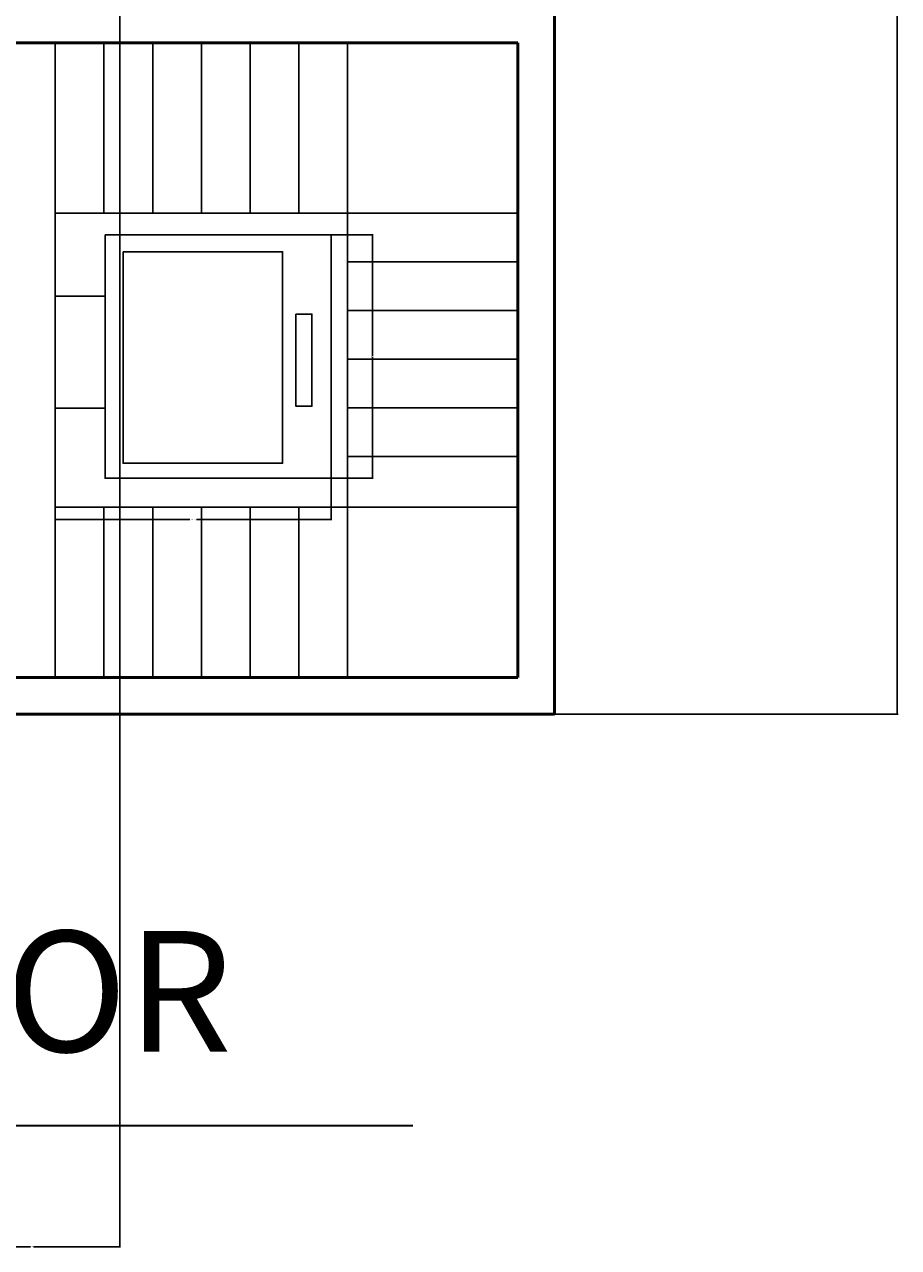
# Model space of a CAD drawing. Units: inches. Extents: x 7359 to 7979, y 33027 to 34263.
# Tile 17 of 32: x 7764 to 7979, y 33027 to 33329. Entities that reach past the tile are written whole.
import ezdxf

# ---------------------------------------------------------------- set-up
doc = ezdxf.new("R2010")
doc.units = ezdxf.units.IN
for name, color, linetype, lineweight in [('A-ANNO-DIMS', 2, 'Continuous', 18), ('A-ANNO-TITL', 7, 'Continuous', 35), ('A-CONV', 6, 'Continuous', 25), ('A-FLOR-STRS', 7, 'Continuous', 25), ('A-WALL', 7, 'Continuous', 50)]:
    doc.layers.add(name, color=color, linetype=linetype, lineweight=lineweight)
doc.styles.get("Standard").update_dxf_attribs({"font": 'arial.ttf'})
doc.dimstyles.get("Standard").update_dxf_attribs({"dimtxt": 0.18, "dimasz": 0.18, "dimexe": 0.18, "dimexo": 0.0625, "dimgap": 0.09, "dimtad": 0, "dimtih": 1, "dimtoh": 1, "dimdec": 4, "dimzin": 0, "dimdsep": 46, "dimtxsty": 'Standard', "dimcen": 0.09, "dimadec": 0, "dimazin": 0, "dimtfac": 1, "dimtdec": 4, "dimtofl": 0, "dimtmove": 0, "dimatfit": 3, "dimfxl": 1, "dimtolj": 1, "dimtzin": 0, "dimarcsym": 0})

# ---------------------------------------------------------------- blocks, each defined once
blk = doc.blocks.new('STAIR-THREE-FLIGHT')
for p, q in [((0, 156.5), (0, 114.5)), ((12, 156.5), (12, 114.5)), ((24, 156.5), (24, 114.5)), ((36, 156.5), (36, 114.5)), ((48, 156.5), (48, 114.5)), ((60, 156.5), (60, 114.5)), ((72, 156.5), (72, 0)), ((0, 114.5), (114, 114.5)), ((0, 114.5), (0, 42)), ((72, 102.5), (114, 102.5)), ((72, 90.5), (114, 90.5)), ((72, 78.5), (114, 78.5)), ((72, 66.5), (114, 66.5)), ((72, 54.5), (114, 54.5)), ((0, 42), (114, 42)), ((0, 42), (0, 0)), ((12, 42), (12, 0)), ((24, 42), (24, 0)), ((36, 42), (36, 0)), ((48, 42), (48, 0)), ((60, 42), (60, 0))]:
    blk.add_line(p, q)
blk = doc.blocks.new('LIFT-PLAN')
for p, q in [((0, 44.9), (12.25, 44.9)), ((0, 17.24), (12.25, 17.24))]:
    blk.add_line(p, q)
for points in [[(12.25, 60.03), (67.98, 60.03), (67.98, 0), (12.25, 0)], [(16.72, 55.81), (56.03, 55.81), (56.03, 3.68), (16.72, 3.68)], [(59.32, 40.45), (63.26, 40.45), (63.26, 17.73), (59.32, 17.73)]]:
    blk.add_lwpolyline(points, close=True)
blk = doc.blocks.new('*D52')
at = {"layer": 'A-ANNO-DIMS', "color": 0, "lineweight": -2, "transparency": 16777216}
for p, q in [((7771.13, 33216.75), (7771.13, 33206.44)), ((7839.11, 33216.75), (7839.11, 33206.44)), ((7771.31, 33206.62), (7804.3, 33206.62)), ((7838.93, 33206.62), (7805.94, 33206.62))]:
    blk.add_line(p, q, dxfattribs=at)
at = {"layer": 'A-ANNO-DIMS', "color": 0, "transparency": 16777216}
for points in [[(7771.31, 33206.65), (7771.31, 33206.59), (7771.13, 33206.62)], [(7838.93, 33206.65), (7838.93, 33206.59), (7839.11, 33206.62)]]:
    blk.add_solid(points, dxfattribs=at)
at = {"layer": 'Defpoints', "color": 0, "transparency": 16777216}
for p in [(7771.13, 33216.81), (7839.11, 33216.81), (7839.11, 33206.62)]:
    blk.add_point(p, dxfattribs=at)
at = {"layer": 'A-ANNO-DIMS', "color": 0, "transparency": 16777216, "insert": (7805.12, 33206.62), "char_height": 0.18, "attachment_point": 5}
blk.add_mtext('\\A1;LIFT 68 TYP.', dxfattribs=at)
blk = doc.blocks.new('*D53')
at = {"layer": 'A-ANNO-DIMS', "color": 0, "lineweight": -2, "transparency": 16777216}
for p, q in [((7839.17, 33276.84), (7849.49, 33276.84)), ((7849.31, 33276.66), (7849.31, 33247.01)), ((7849.31, 33216.99), (7849.31, 33246.65)), ((7839.17, 33216.81), (7849.49, 33216.81))]:
    blk.add_line(p, q, dxfattribs=at)
at = {"layer": 'A-ANNO-DIMS', "color": 0, "transparency": 16777216}
for points in [[(7849.28, 33276.66), (7849.34, 33276.66), (7849.31, 33276.84)], [(7849.28, 33216.99), (7849.34, 33216.99), (7849.31, 33216.81)]]:
    blk.add_solid(points, dxfattribs=at)
at = {"layer": 'Defpoints', "color": 0, "transparency": 16777216}
for p in [(7839.11, 33276.84), (7849.31, 33276.84), (7839.11, 33216.81)]:
    blk.add_point(p, dxfattribs=at)
at = {"layer": 'A-ANNO-DIMS', "color": 0, "transparency": 16777216, "insert": (7849.31, 33246.83), "char_height": 0.18, "attachment_point": 5}
blk.add_mtext('\\A1;60 TYP.', dxfattribs=at)
blk = doc.blocks.new('*D67')
at = {"layer": 'A-ANNO-DIMS', "color": 0, "lineweight": -2, "transparency": 16777216}
for p, q in [((7894.19, 33627.16), (7978.82, 33627.16)), ((7978.64, 33626.98), (7978.64, 33393.09)), ((7978.64, 33158.84), (7978.64, 33392.73)), ((7894.19, 33158.66), (7978.82, 33158.66))]:
    blk.add_line(p, q, dxfattribs=at)
at = {"layer": 'A-ANNO-DIMS', "color": 0, "transparency": 16777216}
for points in [[(7978.61, 33626.98), (7978.67, 33626.98), (7978.64, 33627.16)], [(7978.61, 33158.84), (7978.67, 33158.84), (7978.64, 33158.66)]]:
    blk.add_solid(points, dxfattribs=at)
at = {"layer": 'Defpoints', "color": 0, "transparency": 16777216}
for p in [(7894.13, 33627.16), (7978.64, 33627.16), (7894.13, 33158.66)]:
    blk.add_point(p, dxfattribs=at)
at = {"layer": 'A-ANNO-DIMS', "color": 0, "transparency": 16777216, "insert": (7978.64, 33392.91), "char_height": 0.18, "attachment_point": 5}
blk.add_mtext('\\A1;468.5', dxfattribs=at)
blk = doc.blocks.new('*D74')
at = {"layer": 'A-ANNO-DIMS', "color": 0, "lineweight": -2, "transparency": 16777216}
for p, q in [((7743.73, 33618.1), (7743.73, 33027.18)), ((7787.03, 33618.1), (7787.03, 33027.18)), ((7743.91, 33027.36), (7765, 33027.36)), ((7786.85, 33027.36), (7765.76, 33027.36))]:
    blk.add_line(p, q, dxfattribs=at)
at = {"layer": 'A-ANNO-DIMS', "color": 0, "transparency": 16777216}
for points in [[(7743.91, 33027.39), (7743.91, 33027.33), (7743.73, 33027.36)], [(7786.85, 33027.39), (7786.85, 33027.33), (7787.03, 33027.36)]]:
    blk.add_solid(points, dxfattribs=at)
at = {"layer": 'Defpoints', "color": 0, "transparency": 16777216}
for p in [(7743.73, 33618.16), (7787.03, 33618.16), (7787.03, 33027.36)]:
    blk.add_point(p, dxfattribs=at)
at = {"layer": 'A-ANNO-DIMS', "color": 0, "transparency": 16777216, "insert": (7765.38, 33027.36), "char_height": 0.18, "attachment_point": 5}
blk.add_mtext('\\A1;43.31', dxfattribs=at)

msp = doc.modelspace()

# ---------------------------------------------------------------- linework, layer by layer
at = {"layer": 'A-ANNO-TITL'}
msp.add_line((7520.8378, 33057.2568), (7859.2391, 33057.2568), dxfattribs=at)
at = {"layer": 'A-WALL'}
for p, q in [((7894.1266, 33627.1623), (7894.1266, 33158.6623)), ((7708.6266, 33324.1623), (7885.1266, 33324.1623)), ((7885.1266, 33324.1623), (7885.1266, 33167.6623)), ((7708.6266, 33167.6623), (7885.1266, 33167.6623)), ((7468.7266, 33158.6623), (7894.1266, 33158.6623))]:
    msp.add_line(p, q, dxfattribs=at)

# ---------------------------------------------------------------- block references
at = {"layer": 'A-CONV'}
msp.add_blockref('LIFT-PLAN', (7771.1261, 33216.8134), dxfattribs=at)
at = {"layer": 'A-FLOR-STRS'}
msp.add_blockref('STAIR-THREE-FLIGHT', (7771.1261, 33167.6624), dxfattribs=at)

# ---------------------------------------------------------------- texts
at = {"layer": 'A-ANNO-TITL'}
msp.add_text('SECOND FLOOR', height=29.769676, dxfattribs=at).set_placement((7513.5868, 33075.4364))

# ---------------------------------------------------------------- dimensions: what is measured, and where the dimension line sits
at = {"layer": 'A-ANNO-DIMS'}
dim = msp.add_linear_dim(base=(7978.6371, 33627.1623), p1=(7894.1266, 33158.6623), p2=(7894.1266, 33627.1623), angle=90, dimstyle='Standard', override={"dimdec": 1, "dimlfac": 1, "dimrnd": 0, "dimzin": 0, "dimdsep": 46, "dimlunit": 2}, dxfattribs=at)
dim.commit()
dim.dimension.update_dxf_attribs({"geometry": '*D67', "text_midpoint": (7978.6371, 33392.9123)})
dim = msp.add_linear_dim(base=(7787.0342, 33027.3568), p1=(7743.7266, 33618.1623), p2=(7787.0342, 33618.1623), dimstyle='Standard', override={"dimdec": 2, "dimlfac": 1, "dimrnd": 0, "dimzin": 0, "dimdsep": 46, "dimlunit": 2}, dxfattribs=at)
dim.commit()
dim.dimension.update_dxf_attribs({"geometry": '*D74', "text_midpoint": (7765.3804, 33027.3568)})
dim = msp.add_linear_dim(base=(7849.3071, 33276.844), p1=(7839.1097, 33216.8138), p2=(7839.1097, 33276.844), angle=90, text='<> TYP.', dimstyle='Standard', override={"dimdec": 0, "dimlfac": 1, "dimrnd": 0, "dimzin": 0, "dimdsep": 46, "dimlunit": 2}, dxfattribs=at)
dim.commit()
dim.dimension.update_dxf_attribs({"geometry": '*D53', "text_midpoint": (7849.3071, 33246.8289)})
dim = msp.add_linear_dim(base=(7839.1097, 33206.6164), p1=(7771.1266, 33216.8138), p2=(7839.1097, 33216.8138), text='LIFT <> TYP.', dimstyle='Standard', override={"dimdec": 0, "dimlfac": 1, "dimrnd": 0, "dimzin": 0, "dimdsep": 46, "dimlunit": 2}, dxfattribs=at)
dim.commit()
dim.dimension.update_dxf_attribs({"geometry": '*D52', "text_midpoint": (7805.1181, 33206.6164)})

doc.saveas('drawing.dxf')
